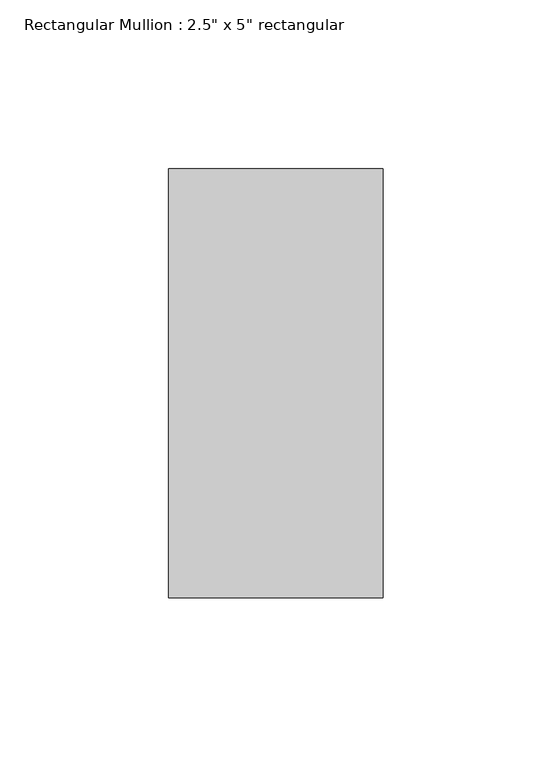
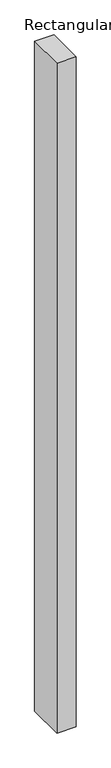
"""IFC4 building model written with IfcOpenShell, lengths in millimetres: member geometry."""

from ifc_helpers import new_model, si_unit, frame, origin, place, context, project, spatial, polyline, outline, extrude, source, transform, mapped, element, save


def member_eadc486f(model_context):
    return source(origin(), model_context, "Body", "SweptSolid", [
        extrude(outline(polyline([(0.0, 63.5), (0.0, -63.5), (-63.5, -63.5), (-63.5, 63.5), (0.0, 63.5)])), frame((0.0, 0.0, -2343.15), z_axis=(0.0, 0.0, 1.0), x_axis=(1.0, 0.0, 0.0)), (0.0, 0.0, 1.0), 2343.15),
    ])


if __name__ == "__main__":
    model = new_model("IFC4")
    model_context = context("Model", 3, world=origin())
    ifc_project = project(units=[si_unit("LENGTHUNIT", "METRE", prefix="MILLI")], contexts=[model_context])
    site = spatial("IfcSite", under=ifc_project)
    building = spatial("IfcBuilding", under=site)
    placement = place(None, origin())
    member_shape = member_eadc486f(model_context)
    element("IfcMember", 1, ObjectType="Rectangular Mullion : 2.5\" x 5\" rectangular", at=placement, inside=building, context=model_context, shape_type="MappedRepresentation", body=[
        mapped(member_shape, transform((0.0, 0.0, 0.0), x_axis=(1.0, 0.0, 0.0), y_axis=(0.0, 1.0, 0.0), z_axis=(0.0, 0.0, 1.0))),
    ])
    save(model, "model.ifc")

# Revit data of these elements
# Type "Rectangular Mullion : 2.5\" x 5\" rectangular"
#   built-in parameter 1007304 = 0.416667 (stored number, unit not read)
#   built-in parameter 1007301 = 0.104167 (stored number, unit not read)
#   built-in parameter 1007300 = 0.104167 (stored number, unit not read)
# Element 1 (IfcMember, "Rectangular Mullion : 2.5\" x 5\" rectangular")
#   Materials on its faces: "Aluminum"
# Materials
#   "Aluminum": class "Metal", colour RGB 247 247 247, transparency 0, Description = "Aluminum 6061", Cost = 0
